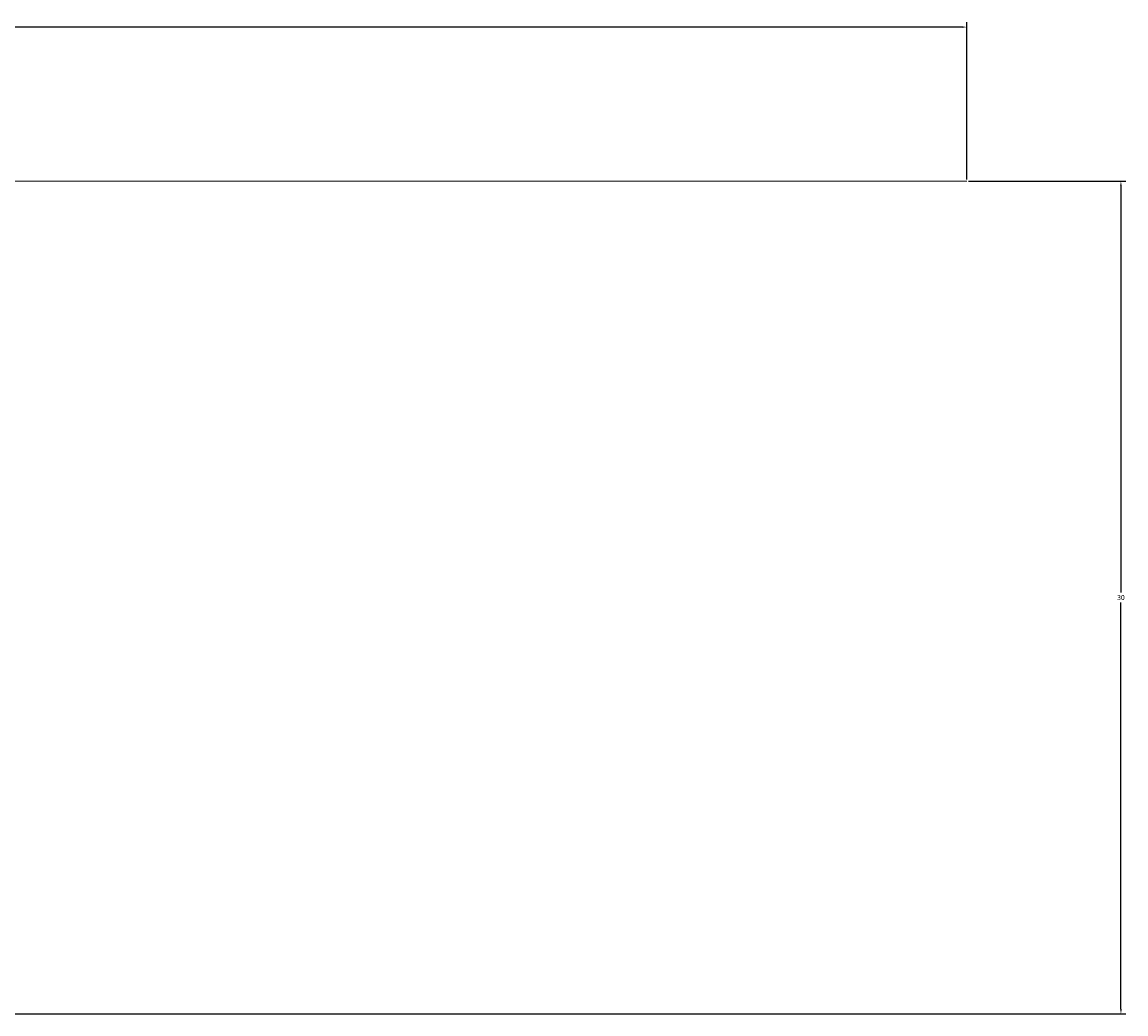
# Model space of a CAD drawing. Units: millimetres. Extents: x 88 to 204, y -56 to 6.
# Tile 3 of 3: x 165 to 204, y -30 to 6. Entities that reach past the tile are written whole.
import ezdxf

# ---------------------------------------------------------------- set-up
doc = ezdxf.new("R2010")
doc.units = ezdxf.units.MM
doc.layers.add('M-CONS', color=8, linetype='Continuous', lineweight=13)
doc.layers.add('M-DIMS', color=2, linetype='Continuous', lineweight=18)
doc.styles.get("Standard").update_dxf_attribs({"font": 'arial.ttf'})
doc.dimstyles.get("Standard").update_dxf_attribs({"dimtxt": 0.18, "dimasz": 0.18, "dimexe": 0.18, "dimexo": 0.0625, "dimgap": 0.09, "dimtad": 0, "dimtih": 1, "dimtoh": 1, "dimdec": 4, "dimzin": 0, "dimdsep": 46, "dimtxsty": 'Standard', "dimcen": 0.09, "dimadec": 0, "dimazin": 0, "dimtfac": 1, "dimtdec": 4, "dimtofl": 0, "dimtmove": 0, "dimatfit": 3, "dimfxl": 1, "dimtolj": 1, "dimtzin": 0, "dimarcsym": 0})

# ---------------------------------------------------------------- blocks, each defined once
blk = doc.blocks.new('*D1')
at = {"layer": 'Defpoints', "color": 0, "transparency": 16777216}
for p in [(198.717, 5.55), (93.717, 0), (198.717, 0)]:
    blk.add_point(p, dxfattribs=at)
at = {"layer": 'M-DIMS', "color": 0, "lineweight": -2, "transparency": 16777216}
for p, q in [((93.717, 0.062), (93.717, 5.73)), ((198.717, 0.062), (198.717, 5.73)), ((93.897, 5.55), (145.936, 5.55)), ((198.537, 5.55), (146.498, 5.55))]:
    blk.add_line(p, q, dxfattribs=at)
at = {"layer": 'M-DIMS', "color": 0, "transparency": 16777216}
for points in [[(93.897, 5.58), (93.897, 5.52), (93.717, 5.55)], [(198.537, 5.58), (198.537, 5.52), (198.717, 5.55)]]:
    blk.add_solid(points, dxfattribs=at)
at = {"layer": 'M-DIMS', "color": 0, "transparency": 16777216, "insert": (146.217, 5.55), "char_height": 0.18, "attachment_point": 5}
blk.add_mtext('\\A1;105', dxfattribs=at)
blk = doc.blocks.new('*D6')
at = {"layer": 'Defpoints', "color": 0, "transparency": 16777216}
for p in [(198.717, 0), (163.717, -30), (204.267, -30)]:
    blk.add_point(p, dxfattribs=at)
at = {"layer": 'M-DIMS', "color": 0, "lineweight": -2, "transparency": 16777216}
for p, q in [((198.779, 0), (204.447, 0)), ((204.267, -0.18), (204.267, -14.818)), ((204.267, -29.82), (204.267, -15.182)), ((163.779, -30), (204.447, -30))]:
    blk.add_line(p, q, dxfattribs=at)
at = {"layer": 'M-DIMS', "color": 0, "transparency": 16777216}
for points in [[(204.237, -0.18), (204.297, -0.18), (204.267, 0)], [(204.237, -29.82), (204.297, -29.82), (204.267, -30)]]:
    blk.add_solid(points, dxfattribs=at)
at = {"layer": 'M-DIMS', "color": 0, "transparency": 16777216, "insert": (204.267, -15), "char_height": 0.18, "attachment_point": 5}
blk.add_mtext('\\A1;30', dxfattribs=at)

msp = doc.modelspace()

# ---------------------------------------------------------------- linework, layer by layer
at = {"layer": 'M-CONS', "extrusion": (0, -1, 0)}
for p, q in [((133.717, 0, 152.588), (198.717, 0, 152.588)), ((198.717, 0, 102.588), (188.717, 0, 102.588))]:
    msp.add_line(p, q, dxfattribs=at)

# ---------------------------------------------------------------- dimensions: what is measured, and where the dimension line sits
at = {"layer": 'M-DIMS'}
dim = msp.add_linear_dim(base=(198.717, 5.55), p1=(93.717, 0), p2=(198.717, 0), dimstyle='Standard', override={"dimdec": 0, "dimlfac": 1, "dimrnd": 0, "dimzin": 0, "dimdsep": 46, "dimlunit": 2}, dxfattribs=at)
dim.commit()
dim.dimension.update_dxf_attribs({"geometry": '*D1', "text_midpoint": (146.217, 5.55)})
dim = msp.add_linear_dim(base=(204.267, -30), p1=(198.717, 0), p2=(163.717, -30), angle=90, dimstyle='Standard', override={"dimdec": 0, "dimlfac": 1, "dimrnd": 0, "dimzin": 0, "dimdsep": 46, "dimlunit": 2}, dxfattribs=at)
dim.commit()
dim.dimension.update_dxf_attribs({"geometry": '*D6', "text_midpoint": (204.267, -15)})

doc.saveas('drawing.dxf')
